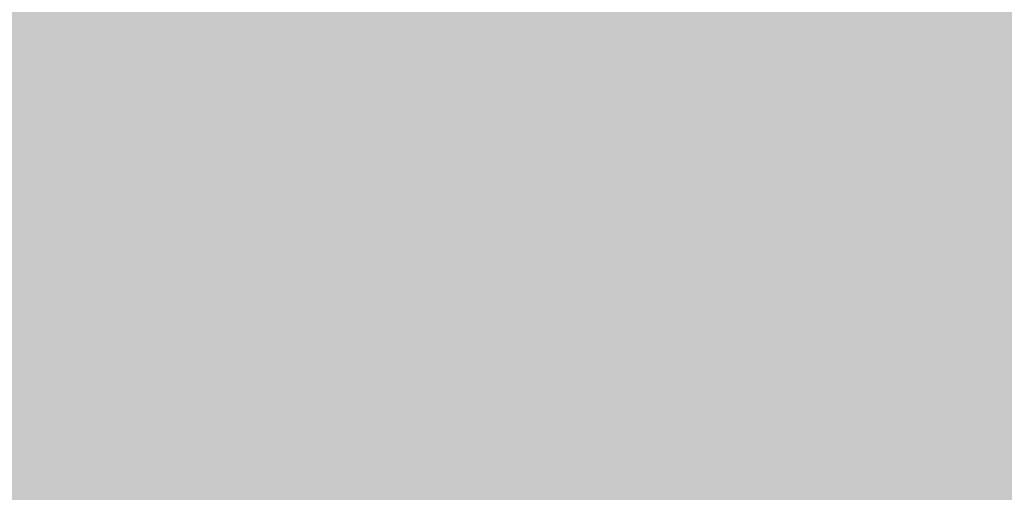
# Model space of a CAD drawing. Units: inches. Extents: x 2083 to 3317, y 1141 to 2115.
# Tile 139 of 256: x 3126.1318 to 3126.6699, y 1263.3548 to 1263.6134. Entities that reach past the tile are written whole.
import ezdxf

# ---------------------------------------------------------------- set-up
doc = ezdxf.new("R2010")
doc.units = ezdxf.units.IN
doc.layers.add('A-ANNO-DIMS', color=2, linetype='Continuous', lineweight=18)
doc.layers.add('A-WALL-PATT', color=251, linetype='Continuous', lineweight=13, true_color=0x636466)
doc.styles.get("Standard").update_dxf_attribs({"font": 'arial.ttf'})
doc.dimstyles.new('ISO-25', dxfattribs={"dimtxt": 12, "dimasz": 12, "dimexe": 1.25, "dimexo": 0.625, "dimtad": 1, "dimlunit": 3, "dimtxsty": 'Standard', "dimcen": 2.5, "dimadec": 0, "dimazin": 0, "dimtfac": 1, "dimtmove": 0, "dimatfit": 3, "dimfxl": 1, "dimarcsym": 0})

# ---------------------------------------------------------------- blocks, each defined once
blk = doc.blocks.new('*D26')
at = {"layer": 'A-ANNO-DIMS', "color": 0, "lineweight": -2, "transparency": 16777216}
for p, q in [((3088.98584, 1274.91509), (3088.98584, 1270.95196)), ((3111.24004, 1274.91509), (3111.24004, 1270.95196)), ((3076.98584, 1272.20196), (2840.26245, 1272.20196)), ((3111.24004, 1272.20196), (3088.98584, 1272.20196)), ((3123.24004, 1272.20196), (3135.24004, 1272.20196))]:
    blk.add_line(p, q, dxfattribs=at)
at = {"layer": 'A-ANNO-DIMS', "color": 0, "transparency": 16777216}
for points in [[(3076.98584, 1274.20196), (3076.98584, 1270.20196), (3088.98584, 1272.20196)], [(3123.24004, 1274.20196), (3123.24004, 1270.20196), (3111.24004, 1272.20196)]]:
    blk.add_solid(points, dxfattribs=at)
at = {"layer": 'Defpoints', "color": 0, "transparency": 16777216}
for p in [(3088.98584, 1275.54009), (3111.24004, 1275.54009), (3088.98584, 1272.20196)]:
    blk.add_point(p, dxfattribs=at)
at = {"layer": 'A-ANNO-DIMS', "color": 0, "transparency": 16777216, "insert": (2952.62415, 1279.0316), "char_height": 12, "attachment_point": 5}
blk.add_mtext('NIGHTSTAND 1\'-10 1/2" TYP.', dxfattribs=at)
blk = doc.blocks.new('*D27')
at = {"layer": 'A-ANNO-DIMS', "color": 0, "lineweight": -2, "transparency": 16777216}
for p, q in [((3114.57817, 1309.79428), (3114.57817, 1321.79428)), ((3111.86504, 1297.79428), (3115.82817, 1297.79428)), ((3114.57817, 1297.79428), (3114.57817, 1275.54009)), ((3111.86504, 1275.54009), (3115.82817, 1275.54009)), ((3114.57817, 1263.54009), (3114.57817, 1140.98859))]:
    blk.add_line(p, q, dxfattribs=at)
at = {"layer": 'A-ANNO-DIMS', "color": 0, "transparency": 16777216}
for points in [[(3112.57817, 1309.79428), (3116.57817, 1309.79428), (3114.57817, 1297.79428)], [(3112.57817, 1263.54009), (3116.57817, 1263.54009), (3114.57817, 1275.54009)]]:
    blk.add_solid(points, dxfattribs=at)
at = {"layer": 'Defpoints', "color": 0, "transparency": 16777216}
for p in [(3111.24004, 1297.79428), (3111.24004, 1275.54009), (3114.57817, 1275.54009)]:
    blk.add_point(p, dxfattribs=at)
at = {"layer": 'A-ANNO-DIMS', "color": 0, "transparency": 16777216, "insert": (3107.74853, 1196.26434), "char_height": 12, "attachment_point": 5, "rotation": 90}
blk.add_mtext('1\'-10 1/2" TYP.', dxfattribs=at)

msp = doc.modelspace()

# ---------------------------------------------------------------- hatches: boundary and pattern name
at = {"layer": 'A-WALL-PATT'}
h = msp.add_hatch(color=256, dxfattribs=at)
h.dxf.hatch_style = 1
h.paths.add_polyline_path([(3126.95978, 2020.76136), (2748.95978, 2020.76136), (2604.95978, 2020.76136), (2226.95978, 2020.76136), (2226.95978, 1702.76136), (2466.95978, 1702.76136), (2466.95978, 1582.76136), (2418.95978, 1582.76136), (2418.95978, 1477.76136), (2226.95978, 1477.76136), (2226.95978, 1263.26136), (2544.95978, 1263.26136), (2544.95978, 1411.76136), (2604.95978, 1411.76136), (2685.95978, 1411.76136), (2685.95978, 1420.76136), (2604.95978, 1420.76136), (2604.95978, 1573.76136), (2604.95978, 1702.76136), (2604.95978, 2011.76136), (2748.95978, 2011.76136), (2748.95978, 1702.76136), (2862.95978, 1702.76136), (2862.95978, 1621.76136), (2871.95978, 1621.76136), (2871.95978, 1702.76136), (2883.95978, 1702.76136), (2883.95978, 1706.93946, -0.026459), (2883.95978, 1711.76136), (2757.95978, 1711.76136), (2757.95978, 1807.76136), (2787.95978, 1807.76136), (2787.95978, 1812.26136), (2757.95978, 1812.26136), (2757.95978, 2011.76136), (2877.95978, 2011.76136), (2877.95978, 1812.26136), (2847.95978, 1812.26136), (2847.95978, 1807.76136), (2889.83574, 1807.76136), (2889.83574, 1812.26136), (2882.45978, 1812.26136), (2882.45978, 2011.76136), (3117.95978, 2011.76136), (3117.95978, 1812.26136), (2937.83574, 1812.26136), (2937.83574, 1807.76136), (2995.70978, 1807.76136), (2995.70978, 1796.11767), (3000.20978, 1796.11767), (3000.20978, 1807.76136), (3117.95978, 1807.76136), (3117.95978, 1711.76136), (3000.20978, 1711.76136), (3000.20978, 1760.11767), (2998.5727, 1760.11767, -0.020711), (2995.70978, 1760.11767), (2995.70978, 1711.76136), (2931.95978, 1711.76136), (2931.95978, 1702.76136), (3126.95978, 1702.76136)])
h.paths.add_polyline_path([(2471.45978, 2011.76136), (2471.45978, 1810.01136), (2462.71694, 1810.01136), (2462.71694, 1805.51136), (2505.95978, 1805.51136), (2505.95978, 1810.01136), (2475.95978, 1810.01136), (2475.95978, 2011.76136), (2595.95978, 2011.76136), (2595.95978, 1810.01136), (2565.95978, 1810.01136), (2565.95978, 1805.51136), (2595.95978, 1805.51136), (2595.95978, 1711.76136), (2235.95978, 1711.76136), (2235.95978, 1805.51136), (2353.70978, 1805.51136), (2353.70978, 1796.05416), (2358.20978, 1796.05416), (2358.20978, 1805.51136), (2414.71694, 1805.51136), (2414.71694, 1810.01136), (2235.95978, 1810.01136), (2235.95978, 2011.76136)], flags=16)
h.paths.add_polyline_path([(2270.20473, 1994.61001), (2270.20473, 1970.61001), (2246.20473, 1970.61001), (2246.20473, 1994.61001)], flags=0)
edge = h.paths.add_edge_path(flags=0)
edge.add_ellipse((2332.02739, 1899.79818), major_axis=(-3.04299, 3.04299), ratio=0.1682525, start_angle=-161.33217, end_angle=-156.30711, ccw=False)
edge.add_ellipse((2333.08204, 1898.74353), major_axis=(-1.05465, 1.05465), ratio=0.4535321, start_angle=-123.37102, end_angle=-94.15911)
edge = h.paths.add_edge_path(flags=0)
edge.add_ellipse((2332.02739, 1968.87629), major_axis=(3.04299, 3.04299), ratio=0.1682525, start_angle=18.66783, end_angle=23.69289)
edge.add_spline(control_points=[(2332.9256, 1970.6911), (2332.22677, 1970.3361), (2330.89371, 1969.65891), (2328.41308, 1970.93214), (2327.20393, 1967.74871), (2324.7096, 1969.95559), (2322.53282, 1967.01235), (2320.01285, 1971.29581), (2317.68031, 1968.15784), (2316.04053, 1967.10205), (2315.4269, 1966.8096)], knot_values=[0, 0, 0, 0, 2.267059, 4.324559, 6.685584, 8.878641, 11.121502, 14.300359, 17.755284, 19.732645, 19.732645, 19.732645, 19.732645], degree=3, periodic=0)
edge.add_ellipse((2332.02739, 1968.87629), major_axis=(3.04299, 3.04299), ratio=0.1682525, start_angle=18.66783, end_angle=23.69289, ccw=False)
edge.add_ellipse((2333.08204, 1969.93094), major_axis=(1.05465, 1.05465), ratio=0.4535321, start_angle=56.62898, end_angle=85.84089, ccw=False)
edge = h.paths.add_edge_path(flags=0)
edge.add_spline(control_points=[(2296.42829, 1967.98791), (2293.6278, 1965.33631), (2287.70362, 1959.72709), (2299.74386, 1949.9957), (2294.53259, 1935.66853), (2290.57323, 1920.60351), (2293.39412, 1909.97369), (2296.18541, 1904.96654)], knot_values=[0.099185, 0.099185, 0.099185, 0.099185, 0.345301, 0.619822, 0.982653, 1.386093, 1.810555, 1.810555, 1.810555, 1.810555], degree=3, periodic=0)
edge.add_spline(control_points=[(2296.18541, 1904.96654), (2297.38358, 1902.6193), (2298.00097, 1901.94931), (2298.55297, 1901.46815)], knot_values=[0.006246, 0.006246, 0.006246, 0.006246, 0.055476, 0.055476, 0.055476, 0.055476], degree=3, periodic=0)
edge.add_spline(control_points=[(2298.55297, 1901.46815), (2297.25861, 1900.92322), (2295.22529, 1900.23213), (2293.06023, 1900.61421), (2292.10142, 1900.78841), (2292.08958, 1900.79057)], knot_values=[0.312835, 0.312835, 0.312835, 0.312835, 0.40178, 0.474987, 0.475903, 0.475903, 0.475903, 0.475903], degree=3, periodic=0)
edge.add_arc((2292.79365, 1904.66411), 3.93701, 215.4209, 259.69818, ccw=False)
edge.add_spline(control_points=[(2289.58531, 1902.3823), (2289.47665, 1902.53509), (2289.36848, 1902.68804), (2289.26086, 1902.84117)], knot_values=[0.102872, 0.102872, 0.102872, 0.102872, 0.116896, 0.116896, 0.116896, 0.116896], degree=3, periodic=0)
edge.add_spline(control_points=[(2289.26086, 1902.84117), (2288.6866, 1902.55019), (2287.64005, 1902.0199), (2285.88134, 1901.87395), (2283.85297, 1901.50435), (2281.71999, 1899.71054), (2278.46699, 1899.49294), (2276.15714, 1901.8832), (2272.25895, 1899.80407), (2267.77761, 1901.84318), (2262.24388, 1900.18403), (2257.41493, 1901.78206), (2254.31837, 1900.72612), (2253.17828, 1900.33734)], knot_values=[0, 0, 0, 0, 1.907977, 3.477176, 5.261074, 7.972851, 11.680248, 13.717921, 16.939592, 22.789562, 27.502503, 33.595215, 37.145618, 37.145618, 37.145618, 37.145618], degree=3, periodic=0)
edge.add_line((2253.17828, 1900.33734), (2250.24424, 1902.84117))
edge.add_line((2250.24424, 1902.84117), (2250.24424, 1965.8333))
edge.add_line((2250.24424, 1965.8333), (2253.17828, 1968.33712))
edge.add_spline(control_points=[(2253.17828, 1968.33712), (2254.31837, 1967.94835), (2257.41493, 1966.89241), (2262.24388, 1968.49043), (2267.77761, 1966.83128), (2271.52673, 1968.53722), (2273.87591, 1967.82829), (2274.2067, 1967.72764)], knot_values=[0, 0, 0, 0, 0.09018, 0.244935, 0.364644, 0.513233, 0.537855, 0.537855, 0.537855, 0.537855], degree=3, periodic=0)
edge.add_arc((2274.35289, 1963.79335), 3.93701, 72.05113, 92.12795, ccw=False)
edge.add_arc((2281.29693, 1985.23), 18.5963, 252.051134, 288.565722)
edge.add_arc((2292.31672, 1956.02888), 12.64608, 71.026788, 113.778218, ccw=False)
edge = h.paths.add_edge_path(flags=0)
edge.add_spline(control_points=[(2274.89941, 1951.85619), (2275.06616, 1951.61659), (2275.23269, 1951.37659), (2275.39799, 1951.13585)], knot_values=[1.409916, 1.409916, 1.409916, 1.409916, 1.43159, 1.43159, 1.43159, 1.43159], degree=3, periodic=0)
edge.add_spline(control_points=[(2275.39799, 1951.13585), (2275.79211, 1950.56189), (2276.17923, 1949.98377), (2276.54555, 1949.3971)], knot_values=[1.358238, 1.358238, 1.358238, 1.358238, 1.409916, 1.409916, 1.409916, 1.409916], degree=3, periodic=0)
edge.add_line((2276.54555, 1949.3971), (2277.43729, 1947.86218))
edge.add_spline(control_points=[(2277.43729, 1947.86218), (2276.30383, 1945.67311), (2274.6397, 1942.42688), (2274.63161, 1938.0939), (2272.79912, 1930.85155), (2274.35643, 1943.89705), (2275.94768, 1947.92336), (2276.54555, 1949.3971)], knot_values=[0.005632, 0.005632, 0.005632, 0.005632, 0.186014, 0.266002, 0.357087, 0.59639, 0.739732, 0.739732, 0.739732, 0.739732], degree=3, periodic=0)
edge.add_spline(control_points=[(2276.54555, 1949.3971), (2276.17923, 1949.98377), (2275.79211, 1950.56189), (2275.39799, 1951.13585)], knot_values=[1.358238, 1.358238, 1.358238, 1.358238, 1.409916, 1.409916, 1.409916, 1.409916], degree=3, periodic=0)
edge.add_spline(control_points=[(2275.39799, 1951.13585), (2274.9425, 1950.08045), (2274.20776, 1948.02527), (2273.9346, 1944.85148), (2272.46853, 1937.62749), (2273.46622, 1945.69647), (2274.70062, 1951.05947), (2274.89941, 1951.85619)], knot_values=[0.104364, 0.104364, 0.104364, 0.104364, 0.189636, 0.269624, 0.36071, 0.600013, 0.644622, 0.644622, 0.644622, 0.644622], degree=3, periodic=0)
h.paths.add_polyline_path([(2269.16751, 1963.12757, -0.357527), (2268.17063, 1960.97637, -0.092561), (2268.17063, 1939.43632, -0.357527), (2269.16751, 1937.28512, -0.357527), (2267.01631, 1938.282, -0.164785), (2254.68558, 1938.282, -0.357527), (2252.53438, 1937.28512, -0.357527), (2253.53126, 1939.43632, -0.092561), (2253.53126, 1960.97637, -0.357527), (2252.53438, 1963.12757, -0.357527), (2254.68558, 1962.13069, -0.164785), (2267.01631, 1962.13069, -0.357527)], flags=0)
h.paths.add_polyline_path([(2248.87407, 1967.8018), (2248.87407, 1957.02771), (2249.45778, 1957.02771), (2249.45778, 1911.64676), (2248.87407, 1911.64676), (2248.87407, 1900.87267), (2246.51186, 1900.87267, 0.197327), (2244.14966, 1902.45687), (2244.14966, 1966.21759, 0.197327), (2246.51186, 1967.8018)], flags=0)
h.paths.add_polyline_path([(2269.16751, 1931.38934, -0.357527), (2268.17063, 1929.23814, -0.092561), (2268.17063, 1907.6981, -0.357527), (2269.16751, 1905.54689, -0.357527), (2267.01631, 1906.54377, -0.164785), (2254.68558, 1906.54377, -0.357527), (2252.53438, 1905.54689, -0.357527), (2253.53126, 1907.6981, -0.092561), (2253.53126, 1929.23814, -0.357527), (2252.53438, 1931.38934, -0.357527), (2254.68558, 1930.39246, -0.164785), (2267.01631, 1930.39246, -0.357527)], flags=0)
edge = h.paths.add_edge_path(flags=0)
edge.add_spline(control_points=[(2276.19686, 1906.7237), (2276.16814, 1909.02893), (2276.11405, 1913.37185), (2270.59842, 1924.92498), (2273.90517, 1919.01278), (2275.92171, 1916.26206), (2275.47457, 1912.40215), (2277.25787, 1910.38062), (2276.69604, 1908.22504), (2276.64622, 1906.81302), (2276.61782, 1906.00841)], knot_values=[0, 0, 0, 0, 8.61026, 16.221274, 18.843057, 23.804898, 27.440828, 29.356102, 31.203478, 33.650687, 33.650687, 33.650687, 33.650687], degree=3, periodic=0)
edge.add_spline(control_points=[(2276.61782, 1906.00841), (2276.62331, 1905.62414), (2276.49774, 1904.62866), (2275.44178, 1903.85473), (2274.93731, 1903.08045), (2274.85908, 1902.84117)], knot_values=[0.156488, 0.156488, 0.156488, 0.156488, 0.184398, 0.231376, 0.250598, 0.250598, 0.250598, 0.250598], degree=3, periodic=0)
edge.add_line((2274.85908, 1902.84117), (2276.50598, 1902.84117))
edge.add_spline(control_points=[(2276.50598, 1902.84117), (2276.78831, 1903.08494), (2277.66507, 1904.1252), (2278.24954, 1904.34074), (2277.65387, 1908.52739), (2278.15567, 1906.22781), (2278.10046, 1905.28595), (2278.84667, 1904.06901), (2277.85679, 1903.41495), (2277.87419, 1902.99105), (2277.90356, 1902.84117)], knot_values=[0.059574, 0.059574, 0.059574, 0.059574, 0.080753, 0.103741, 0.16972, 0.176036, 0.207137, 0.240474, 0.262341, 0.27366, 0.27366, 0.27366, 0.27366], degree=3, periodic=0)
edge.add_line((2277.90356, 1902.84117), (2280.02983, 1902.84117))
edge.add_spline(control_points=[(2280.02983, 1902.84117), (2279.88822, 1903.0884), (2279.49926, 1903.98155), (2280.15228, 1905.93935), (2278.10362, 1909.65776), (2279.76239, 1907.18529), (2280.3279, 1904.87486), (2280.48511, 1903.48959), (2281.46327, 1903.24943), (2281.75834, 1902.9365), (2281.83404, 1902.84117)], knot_values=[0.013856, 0.013856, 0.013856, 0.013856, 0.034874, 0.088867, 0.107879, 0.126738, 0.158714, 0.193757, 0.217487, 0.226722, 0.226722, 0.226722, 0.226722], degree=3, periodic=0)
edge.add_spline(control_points=[(2281.83404, 1902.84117), (2281.78753, 1902.8267), (2281.64702, 1902.78299), (2281.39553, 1902.85949), (2281.08808, 1902.98524), (2280.72068, 1903.0609), (2280.33345, 1903.02573), (2280.12477, 1902.89888), (2280.02983, 1902.84117)], knot_values=[0, 0, 0, 0, 0.14413, 0.435517, 0.749276, 1.153046, 1.548371, 1.878348, 1.878348, 1.878348, 1.878348], degree=3, periodic=0)
edge.add_line((2280.02983, 1902.84117), (2277.90356, 1902.84117))
edge.add_spline(control_points=[(2277.90356, 1902.84117), (2277.89286, 1902.79586), (2277.8654, 1902.67964), (2277.60748, 1902.68748), (2277.27405, 1902.8007), (2276.83792, 1902.61977), (2276.58381, 1902.78926), (2276.50598, 1902.84117)], knot_values=[0, 0, 0, 0, 0.127189, 0.326199, 0.628009, 1.24357, 1.515331, 1.515331, 1.515331, 1.515331], degree=3, periodic=0)
edge.add_line((2276.50598, 1902.84117), (2274.85908, 1902.84117))
edge.add_spline(control_points=[(2274.85908, 1902.84117), (2274.81444, 1902.89859), (2274.72513, 1903.01345), (2274.49348, 1903.11897), (2274.24429, 1902.96054), (2273.93712, 1903.18494), (2273.61404, 1902.98314), (2273.40832, 1902.88304), (2273.32225, 1902.84117)], knot_values=[0, 0, 0, 0, 0.21843, 0.436957, 0.687977, 0.990379, 1.398396, 1.69185, 1.69185, 1.69185, 1.69185], degree=3, periodic=0)
edge.add_spline(control_points=[(2273.32225, 1902.84117), (2273.61674, 1903.44569), (2274.274, 1904.53825), (2276.02724, 1904.5737), (2276.20696, 1906.58364), (2276.19686, 1906.7237)], knot_values=[0.012227, 0.012227, 0.012227, 0.012227, 0.059472, 0.106218, 0.134458, 0.134458, 0.134458, 0.134458], degree=3, periodic=0)
h.paths.add_polyline_path([(2270.77605, 1897.78983), (2270.77605, 1873.78983), (2246.77605, 1873.78983), (2246.77605, 1897.78983)], flags=0)
h.paths.add_polyline_path([(2353.70978, 1760.00506), (2353.70978, 1760.05416), (2358.20978, 1760.05416, -0.033729)], flags=0)
h.paths.add_polyline_path([(2321.81912, 1737.52919), (2341.99533, 1737.52919, -0.414214), (2343.20327, 1736.32124), (2343.20327, 1721.0206, -0.414214), (2341.99533, 1719.81265), (2321.81912, 1719.81265, -0.414214), (2320.61117, 1721.0206), (2320.61117, 1736.32124, -0.414214)], flags=0)
h.paths.add_polyline_path([(2324.23501, 1736.32124), (2339.57944, 1736.32124, -0.414214), (2341.99533, 1733.90535), (2341.99533, 1725.44973, -0.414214), (2339.57944, 1723.03384), (2333.68059, 1723.03384), (2333.84532, 1722.04547, -0.870646), (2335.4254, 1721.82589, -0.767327), (2333.92269, 1721.42324), (2331.29102, 1721.42324, -0.767327), (2329.78832, 1721.82589, -0.870646), (2331.3684, 1722.04547), (2331.53313, 1723.03384), (2324.23501, 1723.03384, -0.414214), (2321.81912, 1725.44973), (2321.81912, 1733.90535, -0.414214)], flags=0)
h.paths.add_polyline_path([(2570.48379, 1928.61544), (2589.68379, 1928.61544), (2590.16883, 1928.61544), (2590.16883, 1904.9934), (2570.48379, 1904.9934)], flags=0)
h.paths.add_polyline_path([(2574.44732, 1927.26382, -1), (2572.82884, 1927.26382, -1)], flags=0)
h.paths.add_polyline_path([(2573.08987, 1926.94088), (2573.92503, 1927.77604), (2574.14774, 1927.55333), (2573.31258, 1926.71817)], flags=0)
h.paths.add_polyline_path([(2578.77906, 1919.72962, -1), (2571.59166, 1919.72962, -1)], flags=0)
h.paths.add_polyline_path([(2578.38536, 1919.72962, -1), (2571.98536, 1919.72962, -1)], flags=0)
h.paths.add_polyline_path([(2331.59576, 1729.47622, -1), (2333.61795, 1729.47622, -1)], flags=0)
h.paths.add_polyline_path([(2578.03423, 1927.26382, -1), (2576.41574, 1927.26382, -1)], flags=0)
h.paths.add_polyline_path([(2576.68885, 1927.53109), (2576.91156, 1927.7538), (2577.74673, 1926.91863), (2577.52402, 1926.69592)], flags=0)
h.paths.add_polyline_path([(2578.13906, 1909.85954, -1), (2572.23166, 1909.85954, -1)], flags=0)
h.paths.add_polyline_path([(2577.74536, 1909.85954, -1), (2572.62536, 1909.85954, -1)], flags=0)
h.paths.add_polyline_path([(2583.79772, 1927.26382, -1), (2582.17923, 1927.26382, -1)], flags=0)
h.paths.add_polyline_path([(2582.71865, 1927.7538), (2583.55381, 1926.91863), (2583.3311, 1926.69592), (2582.49594, 1927.53109)], flags=0)
h.paths.add_polyline_path([(2582.49594, 1927.53109), (2582.71865, 1927.7538), (2583.55381, 1926.91863), (2583.3311, 1926.69592)], flags=0)
h.paths.add_polyline_path([(2587.73906, 1920.52962, -1), (2581.83166, 1920.52962, -1)], flags=0)
h.paths.add_polyline_path([(2587.34536, 1920.52962, -1), (2582.22536, 1920.52962, -1)], flags=0)
h.paths.add_polyline_path([(2587.38462, 1927.26382, -1), (2585.76613, 1927.26382, -1)], flags=0)
h.paths.add_polyline_path([(2586.08199, 1926.98025), (2586.91716, 1927.81541), (2587.13987, 1927.5927), (2586.3047, 1926.75754)], flags=0)
h.paths.add_polyline_path([(2588.37906, 1910.65954, -1), (2581.19166, 1910.65954, -1)], flags=0)
h.paths.add_polyline_path([(2587.98536, 1910.65954, -1), (2581.58536, 1910.65954, -1)], flags=0)
h.paths.add_polyline_path([(2417.16773, 1729.4779), (2437.34394, 1729.4779, -0.414214), (2438.55188, 1728.26995), (2438.55188, 1712.96931, -0.414214), (2437.34394, 1711.76136), (2417.16773, 1711.76136, -0.414214), (2415.95978, 1712.96931), (2415.95978, 1728.26995, -0.414214)], flags=0)
h.paths.add_polyline_path([(2419.58362, 1728.26995), (2434.92805, 1728.26995, -0.414214), (2437.34394, 1725.85406), (2437.34394, 1717.39844, -0.414214), (2434.92805, 1714.98255), (2429.0292, 1714.98255), (2429.19393, 1713.99418, -0.870646), (2430.77401, 1713.7746, -0.767327), (2429.2713, 1713.37195), (2426.63963, 1713.37195, -0.767327), (2425.13693, 1713.7746, -0.870646), (2426.71701, 1713.99418), (2426.88174, 1714.98255), (2419.58362, 1714.98255, -0.414214), (2417.16773, 1717.39844), (2417.16773, 1725.85406, -0.414214)], flags=0)
h.paths.add_polyline_path([(2419.58362, 1728.26995), (2434.92805, 1728.26995, -0.414214), (2437.34394, 1725.85406), (2437.34394, 1717.39844, -0.414214), (2434.92805, 1714.98255), (2429.0292, 1714.98255), (2428.35812, 1719.00903), (2427.55282, 1719.00903), (2426.88174, 1714.98255), (2419.58362, 1714.98255, -0.414214), (2417.16773, 1717.39844), (2417.16773, 1725.85406, -0.414214)], flags=0)
h.paths.add_polyline_path([(2426.94437, 1721.42492, -1), (2428.96656, 1721.42492, -1)], flags=0)
h.paths.add_polyline_path([(2475.95978, 1702.76136), (2595.95978, 1702.76136), (2595.95978, 1582.76136), (2475.95978, 1582.76136)], flags=16)
h.paths.add_polyline_path([(2427.95978, 1573.76136), (2595.95978, 1573.76136), (2595.95978, 1468.76136), (2595.95978, 1420.76136), (2384.45978, 1420.76136), (2384.45978, 1468.76136), (2427.95978, 1468.76136)], flags=16)
h.paths.add_polyline_path([(2379.95978, 1468.76136), (2379.95978, 1420.76136), (2235.95978, 1420.76136), (2235.95978, 1468.76136)], flags=16)
h.paths.add_polyline_path([(2317.816, 1466.69577), (2337.9922, 1466.69577, -0.414214), (2339.20015, 1465.48782), (2339.20015, 1450.18718, -0.414214), (2337.9922, 1448.97923), (2317.816, 1448.97923, -0.414214), (2316.60805, 1450.18718), (2316.60805, 1465.48782, -0.414214)], flags=0)
h.paths.add_polyline_path([(2320.23189, 1465.48782), (2335.57631, 1465.48782, -0.414214), (2337.9922, 1463.07193), (2337.9922, 1454.61631, -0.414214), (2335.57631, 1452.20042), (2329.67747, 1452.20042), (2329.84219, 1451.21205, -0.870646), (2331.42228, 1450.99247, -0.767327), (2329.91957, 1450.58983), (2327.2879, 1450.58983, -0.767327), (2325.7852, 1450.99247, -0.870646), (2327.36528, 1451.21205), (2327.53001, 1452.20042), (2320.23189, 1452.20042, -0.414214), (2317.816, 1454.61631), (2317.816, 1463.07193, -0.414214)], flags=0)
h.paths.add_polyline_path([(2320.23189, 1465.48782), (2335.57631, 1465.48782, -0.414214), (2337.9922, 1463.07193), (2337.9922, 1454.61631, -0.414214), (2335.57631, 1452.20042), (2329.67747, 1452.20042), (2329.00638, 1456.22691), (2328.20109, 1456.22691), (2327.53001, 1452.20042), (2320.23189, 1452.20042, -0.414214), (2317.816, 1454.61631), (2317.816, 1463.07193, -0.414214)], flags=0)
h.paths.add_polyline_path([(2327.59264, 1458.6428, -1), (2329.61483, 1458.6428, -1)], flags=0)
h.paths.add_polyline_path([(2244.41174, 1433.34045), (2241.92094, 1433.34045, -0.414214), (2240.01786, 1435.24354), (2240.01786, 1440.95281, -0.414211), (2241.92093, 1442.8559), (2244.41174, 1442.8559, -1.976472)], flags=0)
h.paths.add_polyline_path([(2245.35689, 1434.39754, -0.414214), (2245.35689, 1441.79881, -2.144098)], flags=0)
h.paths.add_polyline_path([(2535.95978, 1416.26136), (2535.95978, 1272.26136), (2235.95978, 1272.26136), (2235.95978, 1416.26136)], flags=16)
h.paths.add_polyline_path([(2260.11956, 1384.29284), (2260.11956, 1362.03865), (2237.86537, 1362.03865), (2237.86537, 1384.29284)], flags=0)
edge = h.paths.add_edge_path(flags=0)
edge.add_line((2318.25185, 1362.0933), (2318.1458, 1362.00097))
edge.add_ellipse((2317.44512, 1360.43104), major_axis=(2.82164, 2.82164), ratio=0.1682525, start_angle=18.66783, end_angle=20.94813, ccw=False)
edge.add_ellipse((2318.42305, 1361.40897), major_axis=(0.97793, 0.97793), ratio=0.4535321, start_angle=56.62898, end_angle=70.2262, ccw=False)
edge = h.paths.add_edge_path(flags=0)
edge.add_line((2319.10737, 1295.57108), (2319.01504, 1295.67713))
edge.add_ellipse((2317.44512, 1296.37781), major_axis=(-2.82164, 2.82164), ratio=0.1682525, start_angle=-161.33217, end_angle=-159.05187, ccw=False)
edge.add_ellipse((2318.42305, 1295.39988), major_axis=(-0.97793, 0.97793), ratio=0.4535321, start_angle=-123.37102, end_angle=-109.7738)
edge = h.paths.add_edge_path(flags=0)
edge.add_spline(control_points=[(2284.21035, 1301.17022), (2284.58069, 1300.44472), (2284.89119, 1299.89202), (2285.15955, 1299.46102)], knot_values=[0.039066, 0.039066, 0.039066, 0.039066, 0.055476, 0.055476, 0.055476, 0.055476], degree=3, periodic=0)
edge.add_line((2285.15955, 1299.46102), (2284.21035, 1301.17022))
edge = h.paths.add_edge_path(flags=0)
edge.add_line((2280.41246, 1297.29801), (2283.36999, 1297.03612))
edge.add_line((2283.36999, 1297.03612), (2286.40569, 1297.92631))
edge.add_spline(control_points=[(2286.40569, 1297.92631), (2285.30549, 1297.46312), (2284.34478, 1297.12915), (2283.36999, 1297.03612)], knot_values=[0.394369, 0.394369, 0.394369, 0.394369, 0.475903, 0.475903, 0.475903, 0.475903], degree=3, periodic=0)
edge.add_spline(control_points=[(2283.36999, 1297.03612), (2283.28139, 1297.02767), (2282.31629, 1296.95734), (2281.3125, 1297.13448), (2280.42344, 1297.29602), (2280.41246, 1297.29801)], knot_values=[0.312835, 0.312835, 0.312835, 0.312835, 0.320246, 0.393453, 0.394369, 0.394369, 0.394369, 0.394369], degree=3, periodic=0)
edge = h.paths.add_edge_path(flags=0)
edge.add_line((2284.43556, 1359.60729), (2280.44629, 1355.32805))
edge.add_line((2280.44629, 1355.32805), (2279.57999, 1351.01775))
edge.add_line((2279.57999, 1351.01775), (2282.41297, 1346.58043))
edge.add_spline(control_points=[(2282.41297, 1346.58043), (2283.15333, 1345.58924), (2284.2529, 1344.0289), (2284.80104, 1342.38717), (2284.93516, 1341.80554)], knot_values=[1.240098, 1.240098, 1.240098, 1.240098, 1.332892, 1.382712, 1.382712, 1.382712, 1.382712], degree=3, periodic=0)
edge.add_spline(control_points=[(2284.93516, 1341.80554), (2285.31911, 1340.1406), (2285.23303, 1338.4092), (2284.90994, 1336.65412)], knot_values=[1.097484, 1.097484, 1.097484, 1.097484, 1.240098, 1.240098, 1.240098, 1.240098], degree=3, periodic=0)
edge.add_spline(control_points=[(2284.90994, 1336.65412), (2284.58685, 1334.89904), (2284.02675, 1333.12027), (2283.46264, 1331.36058)], knot_values=[0.95487, 0.95487, 0.95487, 0.95487, 1.097484, 1.097484, 1.097484, 1.097484], degree=3, periodic=0)
edge.add_line((2283.46264, 1331.36058), (2281.89038, 1326.15336))
edge.add_line((2281.89038, 1326.15336), (2280.75626, 1321.05609))
edge.add_line((2280.75626, 1321.05609), (2280.2992, 1316.00198))
edge.add_line((2280.2992, 1316.00198), (2280.71593, 1310.95007))
edge.add_line((2280.71593, 1310.95007), (2282.02809, 1305.97214))
edge.add_line((2282.02809, 1305.97214), (2284.21035, 1301.17022))
edge.add_spline(control_points=[(2284.21035, 1301.17022), (2283.34073, 1302.73019), (2282.6119, 1304.33649), (2282.02809, 1305.97214)], knot_values=[0.099185, 0.099185, 0.099185, 0.099185, 0.241799, 0.241799, 0.241799, 0.241799], degree=3, periodic=0)
edge.add_spline(control_points=[(2282.02809, 1305.97214), (2281.44428, 1307.60778), (2281.00549, 1309.27276), (2280.71593, 1310.95007)], knot_values=[0.241799, 0.241799, 0.241799, 0.241799, 0.384413, 0.384413, 0.384413, 0.384413], degree=3, periodic=0)
edge.add_spline(control_points=[(2280.71593, 1310.95007), (2280.43324, 1312.58761), (2280.28939, 1314.27696), (2280.29889, 1315.96203), (2280.2992, 1316.00198)], knot_values=[0.384413, 0.384413, 0.384413, 0.384413, 0.523647, 0.527028, 0.527028, 0.527028, 0.527028], degree=3, periodic=0)
edge.add_spline(control_points=[(2280.2992, 1316.00198), (2280.31233, 1317.68696), (2280.47787, 1319.36793), (2280.75626, 1321.05609)], knot_values=[0.527028, 0.527028, 0.527028, 0.527028, 0.669642, 0.669642, 0.669642, 0.669642], degree=3, periodic=0)
edge.add_spline(control_points=[(2280.75626, 1321.05609), (2281.03465, 1322.74425), (2281.42588, 1324.43961), (2281.89038, 1326.15336)], knot_values=[0.669642, 0.669642, 0.669642, 0.669642, 0.812256, 0.812256, 0.812256, 0.812256], degree=3, periodic=0)
edge.add_spline(control_points=[(2281.89038, 1326.15336), (2282.26438, 1327.53325), (2282.78787, 1329.26181), (2283.35275, 1331.01778), (2283.46264, 1331.36058)], knot_values=[0.812256, 0.812256, 0.812256, 0.812256, 0.927087, 0.95487, 0.95487, 0.95487, 0.95487], degree=3, periodic=0)
edge.add_line((2283.46264, 1331.36058), (2284.90994, 1336.65412))
edge.add_line((2284.90994, 1336.65412), (2284.93516, 1341.80554))
edge.add_line((2284.93516, 1341.80554), (2282.41297, 1346.58043))
edge.add_spline(control_points=[(2282.41297, 1346.58043), (2281.27513, 1348.10379), (2280.07845, 1349.57032), (2279.57999, 1351.01775)], knot_values=[1.382712, 1.382712, 1.382712, 1.382712, 1.525326, 1.525326, 1.525326, 1.525326], degree=3, periodic=0)
edge.add_spline(control_points=[(2279.57999, 1351.01775), (2279.44328, 1351.41472), (2279.13631, 1352.85692), (2279.73519, 1354.29039), (2280.44629, 1355.32805)], knot_values=[1.525326, 1.525326, 1.525326, 1.525326, 1.564439, 1.667941, 1.667941, 1.667941, 1.667941], degree=3, periodic=0)
edge.add_spline(control_points=[(2280.44629, 1355.32805), (2281.42611, 1356.75784), (2282.93084, 1358.18256), (2284.43556, 1359.60729)], knot_values=[1.667941, 1.667941, 1.667941, 1.667941, 1.810555, 1.810555, 1.810555, 1.810555], degree=3, periodic=0)
edge.add_arc((2280.62307, 1348.51818), 11.72618, 71.026788, 113.778218)
edge.add_arc((2270.40489, 1375.59516), 17.24357, 252.051134, 288.565722, ccw=False)
edge.add_arc((2263.96597, 1355.71785), 3.65062, 72.05113, 92.12795)
edge.add_arc((2263.96597, 1355.71785), 3.65062, 92.12795, 177.98513)
edge.add_spline(control_points=[(2260.3176, 1355.8462), (2260.26042, 1354.22067), (2260.55128, 1350.18655), (2262.99934, 1346.76625), (2264.47274, 1344.64902)], knot_values=[1.43159, 1.43159, 1.43159, 1.43159, 1.564144, 1.770695, 1.770695, 1.770695, 1.770695], degree=3, periodic=0)
edge.add_line((2264.47274, 1344.64902), (2264.93559, 1343.98253))
edge.add_spline(control_points=[(2263.80104, 1340.24811), (2263.84324, 1340.51409), (2264.06724, 1341.75647), (2264.51269, 1343.00245), (2264.93505, 1343.98108)], knot_values=[0.53657, 0.53657, 0.53657, 0.53657, 0.559349, 0.644622, 0.644622, 0.644622, 0.644622], degree=3, periodic=0)
edge.add_spline(control_points=[(2264.93505, 1343.98108), (2265.11777, 1343.71497), (2265.29888, 1343.44791), (2265.47676, 1343.17936)], knot_values=[1.384077, 1.384077, 1.384077, 1.384077, 1.409916, 1.409916, 1.409916, 1.409916], degree=3, periodic=0)
edge.add_spline(control_points=[(2265.47676, 1343.17936), (2265.65464, 1342.91082), (2265.8293, 1342.64081), (2265.99913, 1342.36881)], knot_values=[1.358238, 1.358238, 1.358238, 1.358238, 1.384077, 1.384077, 1.384077, 1.384077], degree=3, periodic=0)
edge.add_line((2265.99913, 1342.36881), (2266.82601, 1340.94555))
edge.add_spline(control_points=[(2266.82601, 1340.94555), (2268.8944, 1337.08969), (2271.39817, 1325.843), (2270.51616, 1310.56856), (2275.91938, 1301.86061), (2277.78951, 1299.19945)], knot_values=[0.116896, 0.116896, 0.116896, 0.116896, 0.472987, 1.050969, 1.313793, 1.313793, 1.313793, 1.313793], degree=3, periodic=0)
edge.add_spline(control_points=[(2277.78951, 1299.19945), (2277.83941, 1299.12845), (2277.88943, 1299.0575), (2277.93957, 1298.98658)], knot_values=[0.109884, 0.109884, 0.109884, 0.109884, 0.116896, 0.116896, 0.116896, 0.116896], degree=3, periodic=0)
edge.add_line((2277.93957, 1298.98658), (2277.78885, 1299.19911))
edge.add_spline(control_points=[(2277.78885, 1299.19911), (2277.25658, 1298.92941), (2276.28635, 1298.4379), (2275.03935, 1298.33442), (2274.38333, 1298.2389), (2274.21525, 1298.20934)], knot_values=[33.12187, 33.12187, 33.12187, 33.12187, 35.029056, 36.598255, 37.144827, 37.144827, 37.144827, 37.144827], degree=3, periodic=0)
edge.add_line((2274.21525, 1298.20934), (2273.07315, 1297.89296))
edge.add_spline(control_points=[(2273.07315, 1297.89296), (2272.32294, 1297.57978), (2271.03915, 1296.51051), (2269.24839, 1296.22606), (2268.4231, 1296.37465)], knot_values=[26.532584, 26.532584, 26.532584, 26.532584, 29.198919, 31.839101, 31.839101, 31.839101, 31.839101], degree=3, periodic=0)
edge.add_line((2268.4231, 1296.37465), (2263.8785, 1297.45753))
edge.add_spline(control_points=[(2263.8785, 1297.45753), (2263.55608, 1297.35943), (2261.86031, 1296.83869), (2260.23878, 1297.28241), (2258.93345, 1297.51646)], knot_values=[15.919551, 15.919551, 15.919551, 15.919551, 16.939592, 21.226067, 21.226067, 21.226067, 21.226067], degree=3, periodic=0)
edge.add_line((2258.93345, 1297.51646), (2254.05523, 1297.32901))
edge.add_spline(control_points=[(2254.05523, 1297.32901), (2253.75553, 1297.29582), (2252.11368, 1297.16517), (2250.46187, 1297.54422), (2249.12969, 1297.66788)], knot_values=[5.306517, 5.306517, 5.306517, 5.306517, 6.276435, 10.613034, 10.613034, 10.613034, 10.613034], degree=3, periodic=0)
edge.add_line((2249.12969, 1297.66788), (2244.33165, 1296.87776))
edge.add_line((2244.33165, 1296.87776), (2241.61103, 1299.19945))
edge.add_line((2241.61103, 1299.19945), (2241.61103, 1357.6094))
edge.add_line((2241.61103, 1357.6094), (2244.33165, 1359.9311))
edge.add_line((2244.33165, 1359.9311), (2252.72882, 1359.54269))
edge.add_spline(control_points=[(2252.72882, 1359.54269), (2252.87094, 1359.54644), (2253.30574, 1359.54817), (2253.73984, 1359.51427), (2254.03174, 1359.48243)], knot_values=[0.233291, 0.233291, 0.233291, 0.233291, 0.244935, 0.268927, 0.268927, 0.268927, 0.268927], degree=3, periodic=0)
edge.add_line((2254.03174, 1359.48243), (2259.58719, 1359.41639))
edge.add_spline(control_points=[(2259.58719, 1359.41639), (2260.67707, 1359.6285), (2262.0732, 1359.897), (2263.52369, 1359.45928), (2263.83042, 1359.36595)], knot_values=[0.422516, 0.422516, 0.422516, 0.422516, 0.513233, 0.537855, 0.537855, 0.537855, 0.537855], degree=3, periodic=0)
edge.add_arc((2263.96597, 1355.71785), 3.65062, 72.05113, 92.12795, ccw=False)
edge.add_arc((2270.40489, 1375.59516), 17.24357, 252.051134, 288.565722)
edge.add_arc((2280.62307, 1348.51818), 11.72618, 71.026788, 113.778218, ccw=False)
h.paths.add_polyline_path([(2240.34053, 1359.43471), (2240.34053, 1349.44435), (2240.88178, 1349.44435), (2240.88178, 1307.3645), (2240.34053, 1307.3645), (2240.34053, 1297.37414), (2238.15016, 1297.37414, 0.197327), (2235.95978, 1298.84311), (2235.95978, 1357.96575, 0.197327), (2238.15016, 1359.43471)], flags=0)
h.paths.add_polyline_path([(2259.15779, 1355.1005, -0.357527), (2258.23342, 1353.10578, -0.092561), (2258.23342, 1333.1326, -0.357527), (2259.15779, 1331.13788, -0.357527), (2257.16307, 1332.06225, -0.164785), (2245.7293, 1332.06225, -0.357527), (2243.73458, 1331.13788, -0.357527), (2244.65895, 1333.1326, -0.092561), (2244.65895, 1353.10578, -0.357527), (2243.73458, 1355.1005, -0.357527), (2245.7293, 1354.17613, -0.164785), (2257.16307, 1354.17613, -0.357527)], flags=0)
edge = h.paths.add_edge_path(flags=0)
edge.add_line((2265.99913, 1342.36881), (2266.82601, 1340.94555))
edge.add_line((2266.82601, 1340.94555), (2265.30756, 1337.81407))
edge.add_line((2265.30756, 1337.81407), (2264.35823, 1334.65294))
edge.add_line((2264.35823, 1334.65294), (2264.26201, 1333.7997))
edge.add_spline(control_points=[(2264.26201, 1333.7997), (2264.20836, 1333.18705), (2264.16206, 1332.36553), (2264.00714, 1331.41393), (2263.96905, 1331.20183)], knot_values=[0.464444, 0.464444, 0.464444, 0.464444, 0.516691, 0.531608, 0.531608, 0.531608, 0.531608], degree=3, periodic=0)
edge.add_spline(control_points=[(2263.96905, 1331.20183), (2263.77453, 1330.11887), (2263.42437, 1328.79084), (2263.25742, 1328.53065), (2263.23403, 1328.51461)], knot_values=[0.372682, 0.372682, 0.372682, 0.372682, 0.44885, 0.464444, 0.464444, 0.464444, 0.464444], degree=3, periodic=0)
edge.add_spline(control_points=[(2263.23403, 1328.51461), (2263.09638, 1328.42023), (2263.13117, 1329.30148), (2263.27495, 1330.61575)], knot_values=[0.280919, 0.280919, 0.280919, 0.280919, 0.372682, 0.372682, 0.372682, 0.372682], degree=3, periodic=0)
edge.add_spline(control_points=[(2263.27495, 1330.61575), (2263.41874, 1331.93002), (2263.67152, 1333.67732), (2263.96985, 1335.31503)], knot_values=[0.189157, 0.189157, 0.189157, 0.189157, 0.280919, 0.280919, 0.280919, 0.280919], degree=3, periodic=0)
edge.add_spline(control_points=[(2263.96985, 1335.31503), (2264.1005, 1336.03219), (2264.41878, 1337.62191), (2264.75485, 1338.86443), (2264.94742, 1339.49112)], knot_values=[0.097394, 0.097394, 0.097394, 0.097394, 0.137578, 0.189157, 0.189157, 0.189157, 0.189157], degree=3, periodic=0)
edge.add_spline(control_points=[(2264.94742, 1339.49112), (2265.29002, 1340.60605), (2265.64424, 1341.494), (2265.99913, 1342.36881)], knot_values=[0.005632, 0.005632, 0.005632, 0.005632, 0.097394, 0.097394, 0.097394, 0.097394], degree=3, periodic=0)
h.paths.add_polyline_path([(2259.15779, 1325.67097, -0.357527), (2258.23342, 1323.67625, -0.092561), (2258.23342, 1303.70307, -0.357527), (2259.15779, 1301.70835, -0.357527), (2257.16307, 1302.63272, -0.164785), (2245.7293, 1302.63272, -0.357527), (2243.73458, 1301.70835, -0.357527), (2244.65895, 1303.70307, -0.092561), (2244.65895, 1323.67625, -0.357527), (2243.73458, 1325.67097, -0.357527), (2245.7293, 1324.74661, -0.164785), (2257.16307, 1324.74661, -0.357527)], flags=0)
edge = h.paths.add_edge_path(flags=0)
edge.add_spline(control_points=[(2261.70894, 1317.31142), (2261.67948, 1317.41758), (2261.76186, 1317.38853), (2262.49074, 1316.08987), (2262.96218, 1315.3009)], knot_values=[14.955861, 14.955861, 14.955861, 14.955861, 16.221274, 18.694826, 18.694826, 18.694826, 18.694826], degree=3, periodic=0)
edge.add_spline(control_points=[(2262.96218, 1315.3009), (2262.99044, 1315.25362), (2263.7021, 1314.06738), (2264.34898, 1313.12715), (2264.73005, 1312.16415)], knot_values=[18.694826, 18.694826, 18.694826, 18.694826, 18.843057, 22.433791, 22.433791, 22.433791, 22.433791], degree=3, periodic=0)
edge.add_spline(control_points=[(2264.73005, 1312.16415), (2264.87556, 1311.79644), (2265.17687, 1310.76981), (2265.14307, 1309.55926), (2265.24774, 1308.82419)], knot_values=[22.433791, 22.433791, 22.433791, 22.433791, 23.804898, 26.172756, 26.172756, 26.172756, 26.172756], degree=3, periodic=0)
edge.add_line((2265.24774, 1308.82419), (2265.85077, 1307.17189))
edge.add_spline(control_points=[(2265.85077, 1307.17189), (2266.06502, 1306.82168), (2266.38439, 1306.33225), (2266.4244, 1305.78055), (2266.42037, 1305.61122)], knot_values=[28.062562, 28.062562, 28.062562, 28.062562, 29.356102, 29.911721, 29.911721, 29.911721, 29.911721], degree=3, periodic=0)
edge.add_spline(control_points=[(2266.42037, 1305.61122), (2266.41612, 1305.43259), (2266.394, 1305.25), (2266.36478, 1305.06586)], knot_values=[29.911721, 29.911721, 29.911721, 29.911721, 30.497837, 30.497837, 30.497837, 30.497837], degree=3, periodic=0)
edge.add_line((2266.36478, 1305.06586), (2266.06615, 1302.1363))
edge.add_spline(control_points=[(2266.06615, 1302.1363), (2266.07124, 1301.77998), (2265.99808, 1301.19998), (2265.66327, 1300.75896), (2265.50891, 1300.58588)], knot_values=[0.156488, 0.156488, 0.156488, 0.156488, 0.184398, 0.203543, 0.203543, 0.203543, 0.203543], degree=3, periodic=0)
edge.add_line((2265.50891, 1300.58588), (2264.43534, 1299.19945))
edge.add_line((2264.43534, 1299.19945), (2265.96244, 1299.19945))
edge.add_line((2265.96244, 1299.19945), (2267.33599, 1301.17528))
edge.add_line((2267.33599, 1301.17528), (2267.31167, 1301.98624))
edge.add_spline(control_points=[(2267.31167, 1301.98624), (2267.26111, 1302.8624), (2267.16021, 1303.73713), (2267.27149, 1303.3259)], knot_values=[0.126229, 0.126229, 0.126229, 0.126229, 0.166617, 0.166617, 0.166617, 0.166617], degree=3, periodic=0)
edge.add_spline(control_points=[(2267.27149, 1303.3259), (2267.28003, 1303.2943), (2267.30979, 1303.17537), (2267.37345, 1302.88361), (2267.40612, 1302.68283), (2267.41793, 1302.60103)], knot_values=[0.166617, 0.166617, 0.166617, 0.166617, 0.16972, 0.176036, 0.180765, 0.180765, 0.180765, 0.180765], degree=3, periodic=0)
edge.add_spline(control_points=[(2267.74389, 1300.9875), (2267.68758, 1301.15094), (2267.48052, 1301.65666), (2267.48375, 1302.14479), (2267.41793, 1302.60103)], knot_values=[0.180765, 0.180765, 0.180765, 0.180765, 0.193767, 0.220139, 0.220139, 0.220139, 0.220139], degree=3, periodic=0)
edge.add_line((2267.41793, 1302.60103), (2267.74389, 1300.9875))
edge.add_spline(control_points=[(2267.74389, 1300.9875), (2267.83196, 1300.73188), (2267.93202, 1300.3099), (2267.55484, 1299.97452), (2267.42937, 1299.82921)], knot_values=[0.220139, 0.220139, 0.220139, 0.220139, 0.240474, 0.25489, 0.25489, 0.25489, 0.25489], degree=3, periodic=0)
edge.add_line((2267.42937, 1299.82921), (2267.25836, 1299.19945))
edge.add_line((2267.25836, 1299.19945), (2269.22996, 1299.19945))
edge.add_spline(control_points=[(2269.22996, 1299.19945), (2269.09865, 1299.42869), (2268.84277, 1300.01625), (2269.01157, 1300.91592), (2268.9468, 1301.66074)], knot_values=[0.013856, 0.013856, 0.013856, 0.013856, 0.034874, 0.067073, 0.067073, 0.067073, 0.067073], degree=3, periodic=0)
edge.add_line((2268.9468, 1301.66074), (2268.43158, 1303.60311))
edge.add_spline(control_points=[(2268.43158, 1303.60311), (2268.1756, 1304.19237), (2267.59621, 1305.2513), (2268.0407, 1304.62321), (2268.25139, 1304.28242)], knot_values=[0.090155, 0.090155, 0.090155, 0.090155, 0.107879, 0.120289, 0.120289, 0.120289, 0.120289], degree=3, periodic=0)
edge.add_spline(control_points=[(2268.25139, 1304.28242), (2268.36088, 1304.10533), (2269.05775, 1302.91798), (2269.38269, 1301.59042), (2269.52141, 1300.77593), (2269.57522, 1300.55578)], knot_values=[0.120289, 0.120289, 0.120289, 0.120289, 0.126738, 0.158714, 0.173506, 0.173506, 0.173506, 0.173506], degree=3, periodic=0)
edge.add_line((2269.57522, 1300.55578), (2270.6858, 1299.42126))
edge.add_spline(control_points=[(2270.6858, 1299.42126), (2270.76722, 1299.35725), (2270.83785, 1299.2814), (2270.90292, 1299.19945)], knot_values=[0.21816, 0.21816, 0.21816, 0.21816, 0.226722, 0.226722, 0.226722, 0.226722], degree=3, periodic=0)
edge.add_line((2270.9372, 1299.19291), (2270.90292, 1299.19945))
edge.add_spline(control_points=[(2270.90292, 1299.19945), (2270.85981, 1299.18603), (2270.72951, 1299.1455), (2270.49631, 1299.21644), (2270.27166, 1299.30832), (2270.12102, 1299.34796), (2270.06334, 1299.35956)], knot_values=[0.939174, 0.939174, 0.939174, 0.939174, 1.083304, 1.374691, 1.68845, 1.878348, 1.878348, 1.878348, 1.878348], degree=3, periodic=0)
edge.add_line((2270.06334, 1299.35956), (2269.22996, 1299.19945))
edge.add_line((2269.22996, 1299.19945), (2267.25836, 1299.19945))
edge.add_spline(control_points=[(2267.25836, 1299.19945), (2267.24843, 1299.15743), (2267.22297, 1299.04967), (2266.98382, 1299.05694), (2266.80921, 1299.11623), (2266.6769, 1299.10909), (2266.63653, 1299.10481)], knot_values=[0.757665, 0.757665, 0.757665, 0.757665, 0.884854, 1.083864, 1.385675, 1.515331, 1.515331, 1.515331, 1.515331], degree=3, periodic=0)
edge.add_spline(control_points=[(2266.63653, 1299.10481), (2266.48522, 1299.08879), (2266.23581, 1299.01712), (2266.03461, 1299.15132), (2265.96244, 1299.19945)], knot_values=[0, 0, 0, 0, 0.485905, 0.757665, 0.757665, 0.757665, 0.757665], degree=3, periodic=0)
edge.add_line((2265.96244, 1299.19945), (2264.43534, 1299.19945))
edge.add_line((2264.43534, 1299.19945), (2263.85844, 1299.36712))
edge.add_spline(control_points=[(2263.85844, 1299.36712), (2263.81894, 1299.37091), (2263.77953, 1299.38572), (2263.74013, 1299.4015)], knot_values=[0.845925, 0.845925, 0.845925, 0.845925, 0.978627, 0.978627, 0.978627, 0.978627], degree=3, periodic=0)
edge.add_line((2263.72179, 1299.39643), (2263.01031, 1299.19945))
edge.add_spline(control_points=[(2263.01031, 1299.19945), (2263.24579, 1299.68286), (2263.50603, 1300.12811), (2263.87349, 1300.40803)], knot_values=[0.012227, 0.012227, 0.012227, 0.012227, 0.052971, 0.052971, 0.052971, 0.052971], degree=3, periodic=0)
edge.add_spline(control_points=[(2263.87349, 1300.40803), (2263.93213, 1300.4527), (2264.08424, 1300.55298), (2264.25519, 1300.62422), (2264.35969, 1300.66475)], knot_values=[0.052971, 0.052971, 0.052971, 0.052971, 0.059472, 0.069086, 0.069086, 0.069086, 0.069086], degree=3, periodic=0)
edge.add_line((2264.35969, 1300.66475), (2265.1419, 1301.07777))
edge.add_line((2265.1419, 1301.07777), (2265.67581, 1302.79956))
edge.add_line((2265.67581, 1302.79956), (2265.5407, 1305.70407))
edge.add_line((2265.5407, 1305.70407), (2264.80307, 1309.32772))
edge.add_line((2264.80307, 1309.32772), (2263.04053, 1314.09179))
edge.add_spline(control_points=[(2263.04053, 1314.09179), (2262.38357, 1315.67144), (2261.79597, 1316.99775), (2261.70894, 1317.31142)], knot_values=[11.216896, 11.216896, 11.216896, 11.216896, 14.955861, 14.955861, 14.955861, 14.955861], degree=3, periodic=0)
h.paths.add_polyline_path([(2871.95978, 1416.26136), (2895.91005, 1416.26136), (2895.91005, 1420.76136), (2871.95978, 1420.76136), (2871.95978, 1501.76136), (2862.95978, 1501.76136), (2862.95978, 1420.76136), (2805.95978, 1420.76136), (2805.95978, 1411.76136), (2862.95978, 1411.76136), (2862.95978, 1263.26136), (3126.95978, 1263.26136), (3126.95978, 1411.76136), (3126.95978, 1486.76136), (2943.95978, 1486.76136), (2943.95978, 1477.76136), (2967.86031, 1477.76136), (2967.86031, 1420.76136), (2943.91005, 1420.76136), (2943.91005, 1416.26136), (3117.95978, 1416.26136), (3117.95978, 1420.76136), (2972.36031, 1420.76136), (2972.36031, 1477.76136), (3117.95978, 1477.76136), (3117.95978, 1420.76136), (3117.95978, 1272.26136), (2871.95978, 1272.26136)], flags=0)
h.paths.add_polyline_path([(2457.12563, 1485.94251), (2527.60265, 1485.94251), (2527.60265, 1537.6357), (2457.12563, 1537.6357)], flags=8)
h.paths.add_polyline_path([(2481.00506, 1609.9818), (2590.76582, 1609.9818), (2590.76582, 1682.00336), (2481.00506, 1682.00336)], flags=8)
h.paths.add_polyline_path([(2483.08502, 1729.12678), (2553.56205, 1729.12678), (2553.56205, 1780.81998), (2483.08502, 1780.81998)], flags=8)
h = msp.add_hatch(color=256, dxfattribs=at)
h.dxf.hatch_style = 1
h.paths.add_polyline_path([(3126.95978, 1486.76136), (2943.95978, 1486.76136), (2943.95978, 1477.76136), (2967.86031, 1477.76136), (2967.86031, 1420.76136), (2943.91005, 1420.76136), (2943.91005, 1416.26136), (3117.95978, 1416.26136), (3117.95978, 1420.76136), (2972.36031, 1420.76136), (2972.36031, 1477.76136), (3117.95978, 1477.76136), (3117.95978, 1420.76136), (3117.95978, 1272.26136), (2871.95978, 1272.26136), (2871.95978, 1416.26136), (2895.91005, 1416.26136), (2895.91005, 1420.76136), (2871.95978, 1420.76136), (2871.95978, 1501.76136), (2862.95978, 1501.76136), (2862.95978, 1420.76136), (2805.95978, 1420.76136), (2805.95978, 1411.76136), (2862.95978, 1411.76136), (2862.95978, 1263.26136), (3126.95978, 1263.26136), (3126.95978, 1411.76136)])

# ---------------------------------------------------------------- dimensions: what is measured, and where the dimension line sits
at = {"layer": 'A-ANNO-DIMS'}
for base, p1, p2, angle, text, picture, middle in [((3114.57817, 1275.54009), (3111.24004, 1297.79428), (3111.24004, 1275.54009), 270, '<> TYP.', '*D27', (3107.74853, 1196.26434)), ((3088.98584, 1272.20196), (3111.24004, 1275.54009), (3088.98584, 1275.54009), 180, 'NIGHTSTAND <> TYP.', '*D26', (2952.62415, 1279.0316))]:
    dim = msp.add_linear_dim(base=base, p1=p1, p2=p2, angle=angle, text=text, dimstyle='ISO-25', override={"dimdec": 1, "dimlfac": 1, "dimrnd": 0, "dimzin": 1, "dimdsep": 46, "dimlunit": 4, "dimfrac": 2}, dxfattribs=at)
    dim.commit()
    dim.dimension.update_dxf_attribs({"geometry": picture, "text_midpoint": middle})

doc.saveas('drawing.dxf')
